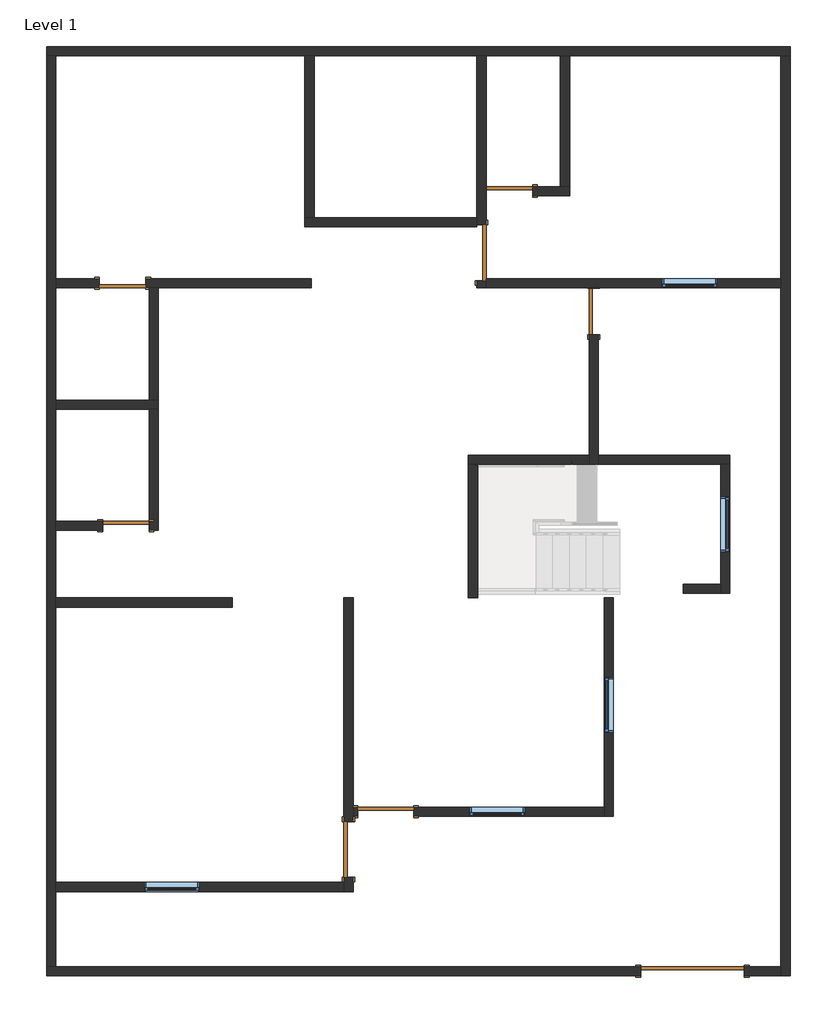
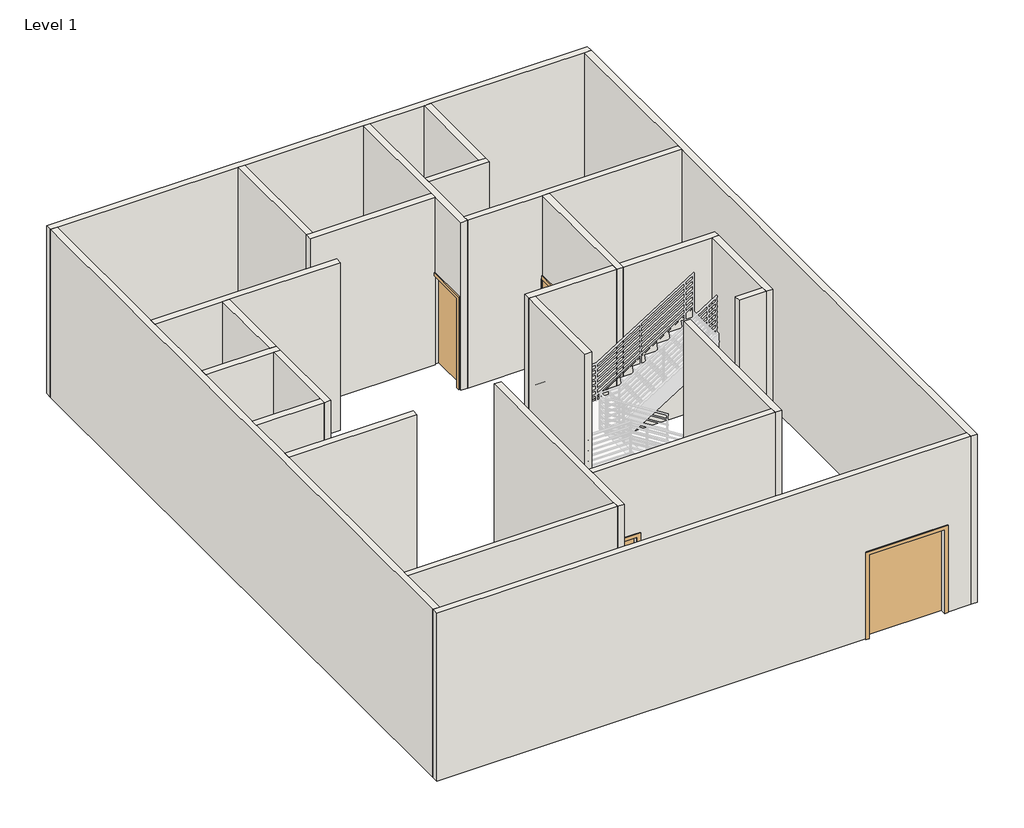
# One storey, part 1 of 4: 26 walls, 8 doors, 5 windows.
"""IFC4 building model written with IfcOpenShell, lengths in millimetres."""

from ifc_helpers import new_model, si_unit, frame, origin, origin_with_axes, place, context, project, spatial, polyline, outline, extrude, faceted_brep, transform, mapped, element, save
from components import m_door_double_flush_panel_double_acting_1700_x_2000mm_42eec5da, m_single_flush_0762_x_2032mm_ffa3ef71, m_single_flush_0762_x_2032mm_3f592dcc, m_single_flush_0915_x_2134mm_138fd904, m_single_flush_0915_x_2134mm_f3d7f739, m_fixed_0915_x_0610mm_ad787ded

model = new_model("IFC4")

# Units and contexts
model_context = context("Model", 3, world=origin())
ifc_project = project(units=[si_unit("LENGTHUNIT", "METRE", prefix="MILLI")], contexts=[model_context])

# Site, building, storey
site = spatial("IfcSite", under=ifc_project)
building = spatial("IfcBuilding", under=site)
storey = spatial("IfcBuildingStorey", under=building, Name="Level 1", Elevation=0.0)

# Doors
placement = place(None, origin())
m_door_double_flush_panel_double_acting_1700_x_2000mm_shape = m_door_double_flush_panel_double_acting_1700_x_2000mm_42eec5da(model_context)
element("IfcDoor", 1, ObjectType="M_Door-Double-Flush_Panel-Double-Acting : 1700 x 2000mm", at=placement, inside=storey, context=model_context, shape_type="MappedRepresentation", body=[
    mapped(m_door_double_flush_panel_double_acting_1700_x_2000mm_shape, transform((658.3084763, -5386.7690536, 0.0), x_axis=(1.0, 0.0, 0.0), y_axis=(0.0, 1.0, 0.0), z_axis=(0.0, 0.0, 1.0))),
])
m_single_flush_0762_x_2032mm_shape = m_single_flush_0762_x_2032mm_ffa3ef71(model_context)
element("IfcDoor", 2, ObjectType="M_Single-Flush : 0762 x 2032mm", at=placement, inside=storey, context=model_context, shape_type="MappedRepresentation", body=[
    mapped(m_single_flush_0762_x_2032mm_shape, transform((-2346.0915237, 7408.1309464, 0.0), x_axis=(-1.0, 0.0, 0.0), y_axis=(0.0, -1.0, 0.0), z_axis=(0.0, 0.0, 1.0))),
])
element("IfcDoor", 3, ObjectType="M_Single-Flush : 0762 x 2032mm", at=placement, inside=storey, context=model_context, shape_type="MappedRepresentation", body=[
    mapped(m_single_flush_0762_x_2032mm_shape, transform((-8686.1415237, 5894.4309464, 0.0), x_axis=(1.0, 0.0, 0.0), y_axis=(0.0, 1.0, 0.0), z_axis=(0.0, 0.0, 1.0))),
])
m_single_flush_0762_x_2032mm_2_shape = m_single_flush_0762_x_2032mm_3f592dcc(model_context)
element("IfcDoor", 4, ObjectType="M_Single-Flush : 0762 x 2032mm", at=placement, inside=storey, context=model_context, shape_type="MappedRepresentation", body=[
    mapped(m_single_flush_0762_x_2032mm_2_shape, transform((-8635.3415237, 1920.5309464, 0.0), x_axis=(1.0, 0.0, 0.0), y_axis=(0.0, 1.0, 0.0), z_axis=(0.0, 0.0, 1.0))),
])
element("IfcDoor", 5, ObjectType="M_Single-Flush : 0762 x 2032mm", at=placement, inside=storey, context=model_context, shape_type="MappedRepresentation", body=[
    mapped(m_single_flush_0762_x_2032mm_2_shape, transform((-962.9915237, 5437.2309464, 0.0), x_axis=(0.0, 1.0, 0.0), y_axis=(-1.0, 0.0, 0.0), z_axis=(0.0, 0.0, 1.0))),
])
m_single_flush_0915_x_2134mm_shape = m_single_flush_0915_x_2134mm_138fd904(model_context)
element("IfcDoor", 6, ObjectType="M_Single-Flush : 0915 x 2134mm", at=placement, inside=storey, context=model_context, shape_type="MappedRepresentation", body=[
    mapped(m_single_flush_0915_x_2134mm_shape, transform((-2803.2915237, 6396.6809464, 0.0), x_axis=(0.0, -1.0, 0.0), y_axis=(1.0, 0.0, 0.0), z_axis=(0.0, 0.0, 1.0))),
])
m_single_flush_0915_x_2134mm_2_shape = m_single_flush_0915_x_2134mm_f3d7f739(model_context)
element("IfcDoor", 7, ObjectType="M_Single-Flush : 0915 x 2134mm", at=placement, inside=storey, context=model_context, shape_type="MappedRepresentation", body=[
    mapped(m_single_flush_0915_x_2134mm_2_shape, transform((-4982.8915237, -3387.7190536, 0.0), x_axis=(0.0, -1.0, 0.0), y_axis=(1.0, 0.0, 0.0), z_axis=(0.0, 0.0, 1.0))),
])
element("IfcDoor", 8, ObjectType="M_Single-Flush : 0915 x 2134mm", at=placement, inside=storey, context=model_context, shape_type="MappedRepresentation", body=[
    mapped(m_single_flush_0915_x_2134mm_2_shape, transform((-4373.2915237, -2771.7690536, 0.0), x_axis=(-1.0, 0.0, 0.0), y_axis=(0.0, -1.0, 0.0), z_axis=(0.0, 0.0, 1.0))),
])

# Walls
element("IfcWall", 9, ObjectType="Generic - 150mm", at=placement, inside=storey, context=model_context, shape_type="Brep", body=[
    faceted_brep([(-9934.6915237, 9628.2309464, 0.0), (-9784.6915237, 9628.2309464, 0.0), (-5698.8915237, 9628.2309464, 0.0), (-5548.8915237, 9628.2309464, 0.0), (-2878.2915237, 9628.2309464, 0.0), (-2728.2915237, 9628.2309464, 0.0), (-1509.0915237, 9628.2309464, 0.0), (-1359.0915237, 9628.2309464, 0.0), (2107.3084763, 9628.2309464, 0.0), (2257.3084763, 9628.2309464, 0.0), (2257.3084763, 9628.2309464, 4000.0), (2107.3084763, 9628.2309464, 4000.0), (-1359.0915237, 9628.2309464, 4000.0), (-1509.0915237, 9628.2309464, 4000.0), (-2728.2915237, 9628.2309464, 4000.0), (-2878.2915237, 9628.2309464, 4000.0), (-5548.8915237, 9628.2309464, 4000.0), (-5698.8915237, 9628.2309464, 4000.0), (-9784.6915237, 9628.2309464, 4000.0), (-9934.6915237, 9628.2309464, 4000.0), (-9934.6915237, 9778.2309464, 0.0), (-9934.6915237, 9778.2309464, 4000.0), (2257.3084763, 9778.2309464, 4000.0), (2257.3084763, 9778.2309464, 0.0)], [[[0, 1, 2, 3, 4, 5, 6, 7, 8, 9, 10, 11, 12, 13, 14, 15, 16, 17, 18, 19]], [[20, 21, 22, 23]], [[9, 8, 7, 6, 5, 4, 3, 2, 1, 0, 20, 23]], [[19, 18, 17, 16, 15, 14, 13, 12, 11, 10, 22, 21]], [[10, 9, 23, 22]], [[0, 19, 21, 20]]]),
])
element("IfcWall", 10, ObjectType="Generic - 150mm", at=placement, inside=storey, context=model_context, shape_type="Brep", body=[
    faceted_brep([(2107.3084763, 9628.2309464, 0.0), (2107.3084763, 5969.4309464, 0.0), (2107.3084763, 5819.4309464, 0.0), (2107.3084763, -5311.7690536, 0.0), (2107.3084763, -5461.7690536, 0.0), (2107.3084763, -5461.7690536, 4000.0), (2107.3084763, -5311.7690536, 4000.0), (2107.3084763, 5819.4309464, 4000.0), (2107.3084763, 5969.4309464, 4000.0), (2107.3084763, 9628.2309464, 4000.0), (2257.3084763, 9628.2309464, 0.0), (2257.3084763, 9628.2309464, 4000.0), (2257.3084763, -5461.7690536, 4000.0), (2257.3084763, -5461.7690536, 0.0)], [[[0, 1, 2, 3, 4, 5, 6, 7, 8, 9]], [[10, 11, 12, 13]], [[4, 3, 2, 1, 0, 10, 13]], [[9, 8, 7, 6, 5, 12, 11]], [[0, 9, 11, 10]], [[5, 4, 13, 12]]]),
])
element("IfcWall", 11, ObjectType="Generic - 150mm", at=placement, inside=storey, context=model_context, shape_type="Brep", body=[
    faceted_brep([(-9934.6915237, -5311.7690536, 4000.0), (-9784.6915237, -5311.7690536, 4000.0), (2107.3084763, -5311.7690536, 4000.0), (2107.3084763, -5311.7690536, 0.0), (1508.3084763, -5311.7690536, 0.0), (1508.3084763, -5311.7690536, 2000.0), (-191.6915237, -5311.7690536, 2000.0), (-191.6915237, -5311.7690536, 0.0), (-9784.6915237, -5311.7690536, 0.0), (-9934.6915237, -5311.7690536, 0.0), (2107.3084763, -5461.7690536, 4000.0), (-9934.6915237, -5461.7690536, 4000.0), (-9934.6915237, -5461.7690536, 0.0), (-191.6915237, -5461.7690536, 0.0), (-191.6915237, -5461.7690536, 2000.0), (1508.3084763, -5461.7690536, 2000.0), (1508.3084763, -5461.7690536, 0.0), (2107.3084763, -5461.7690536, 0.0)], [[[0, 1, 2, 3, 4, 5, 6, 7, 8, 9]], [[10, 11, 12, 13, 14, 15, 16, 17]], [[3, 17, 16, 4]], [[12, 9, 8, 7, 13]], [[2, 1, 0, 11, 10]], [[3, 2, 10, 17]], [[0, 9, 12, 11]], [[15, 5, 4, 16]], [[5, 15, 14, 6]], [[6, 14, 13, 7]]]),
])
element("IfcWall", 12, ObjectType="Generic - 150mm", at=placement, inside=storey, context=model_context, shape_type="Brep", body=[
    faceted_brep([(-9784.6915237, -5311.7690536, 0.0), (-9784.6915237, -4078.6690536, 0.0), (-9784.6915237, -3928.6690536, 0.0), (-9784.6915237, 585.8309464, 0.0), (-9784.6915237, 735.8309464, 0.0), (-9784.6915237, 1845.5309464, 0.0), (-9784.6915237, 1995.5309464, 0.0), (-9784.6915237, 3826.7309464, 0.0), (-9784.6915237, 3976.7309464, 0.0), (-9784.6915237, 5819.4309464, 0.0), (-9784.6915237, 5969.4309464, 0.0), (-9784.6915237, 9628.2309464, 0.0), (-9784.6915237, 9628.2309464, 4000.0), (-9784.6915237, 5969.4309464, 4000.0), (-9784.6915237, 5819.4309464, 4000.0), (-9784.6915237, 3976.7309464, 4000.0), (-9784.6915237, 3826.7309464, 4000.0), (-9784.6915237, 1995.5309464, 4000.0), (-9784.6915237, 1845.5309464, 4000.0), (-9784.6915237, 735.8309464, 4000.0), (-9784.6915237, 585.8309464, 4000.0), (-9784.6915237, -3928.6690536, 4000.0), (-9784.6915237, -4078.6690536, 4000.0), (-9784.6915237, -5311.7690536, 4000.0), (-9934.6915237, -5311.7690536, 0.0), (-9934.6915237, -5311.7690536, 4000.0), (-9934.6915237, 9628.2309464, 4000.0), (-9934.6915237, 9628.2309464, 0.0)], [[[0, 1, 2, 3, 4, 5, 6, 7, 8, 9, 10, 11, 12, 13, 14, 15, 16, 17, 18, 19, 20, 21, 22, 23]], [[24, 25, 26, 27]], [[11, 10, 9, 8, 7, 6, 5, 4, 3, 2, 1, 0, 24, 27]], [[23, 22, 21, 20, 19, 18, 17, 16, 15, 14, 13, 12, 26, 25]], [[12, 11, 27, 26]], [[0, 23, 25, 24]]]),
])
element("IfcWall", 13, ObjectType="Generic - 150mm", at=placement, inside=storey, context=model_context, shape_type="Brep", body=[
    faceted_brep([(-8305.1415237, 5819.4309464, 2032.0), (-8305.1415237, 5819.4309464, 0.0), (-8253.1415237, 5819.4309464, 0.0), (-8103.1415237, 5819.4309464, 0.0), (-5594.8915237, 5819.4309464, 0.0), (-5594.8915237, 5819.4309464, 4000.0), (-8103.1415237, 5819.4309464, 4000.0), (-8253.1415237, 5819.4309464, 4000.0), (-9784.6915237, 5819.4309464, 4000.0), (-9784.6915237, 5819.4309464, 0.0), (-9067.1415237, 5819.4309464, 0.0), (-9067.1415237, 5819.4309464, 2032.0), (-5594.8915237, 5969.4309464, 0.0), (-8305.1415237, 5969.4309464, 0.0), (-8305.1415237, 5969.4309464, 2032.0), (-9067.1415237, 5969.4309464, 2032.0), (-9067.1415237, 5969.4309464, 0.0), (-9784.6915237, 5969.4309464, 0.0), (-9784.6915237, 5969.4309464, 4000.0), (-5594.8915237, 5969.4309464, 4000.0)], [[[0, 1, 2, 3, 4, 5, 6, 7, 8, 9, 10, 11]], [[12, 13, 14, 15, 16, 17, 18, 19]], [[10, 9, 17, 16]], [[4, 3, 2, 1, 13, 12]], [[5, 4, 12, 19]], [[8, 7, 6, 5, 19, 18]], [[9, 8, 18, 17]], [[14, 13, 1, 0]], [[15, 14, 0, 11]], [[16, 15, 11, 10]]]),
])
element("IfcWall", 14, ObjectType="Generic - 150mm", at=placement, inside=storey, context=model_context, shape_type="Brep", body=[
    faceted_brep([(-5698.8915237, 6823.9309464, 0.0), (-2878.2915237, 6823.9309464, 0.0), (-2878.2915237, 6823.9309464, 4000.0), (-5698.8915237, 6823.9309464, 4000.0), (-5698.8915237, 6973.9309464, 0.0), (-5698.8915237, 6973.9309464, 4000.0), (-5548.8915237, 6973.9309464, 4000.0), (-2878.2915237, 6973.9309464, 4000.0), (-2878.2915237, 6973.9309464, 0.0), (-5548.8915237, 6973.9309464, 0.0), (-2878.2915237, 6854.1809464, 0.0)], [[[0, 1, 2, 3]], [[4, 5, 6, 7, 8, 9]], [[1, 0, 4, 9, 8, 10]], [[3, 2, 7, 6, 5]], [[2, 1, 10, 8, 7]], [[0, 3, 5, 4]]]),
])
element("IfcWall", 15, ObjectType="Generic - 150mm", at=placement, inside=storey, context=model_context, shape_type="Brep", body=[
    faceted_brep([(-2728.2915237, 5819.4309464, 0.0), (-2728.2915237, 5939.1809464, 0.0), (-2728.2915237, 5939.1809464, 2134.0), (-2728.2915237, 6854.1809464, 2134.0), (-2728.2915237, 6854.1809464, 0.0), (-2728.2915237, 7333.1309464, 0.0), (-2728.2915237, 7483.1309464, 0.0), (-2728.2915237, 9628.2309464, 0.0), (-2728.2915237, 9628.2309464, 4000.0), (-2728.2915237, 7483.1309464, 4000.0), (-2728.2915237, 7333.1309464, 4000.0), (-2728.2915237, 5969.4309464, 4000.0), (-2728.2915237, 5819.4309464, 4000.0), (-2878.2915237, 5939.1809464, 2134.0), (-2878.2915237, 5939.1809464, 0.0), (-2878.2915237, 5819.4309464, 0.0), (-2878.2915237, 5819.4309464, 4000.0), (-2878.2915237, 6823.9309464, 4000.0), (-2878.2915237, 6973.9309464, 4000.0), (-2878.2915237, 9628.2309464, 4000.0), (-2878.2915237, 9628.2309464, 0.0), (-2878.2915237, 6973.9309464, 0.0), (-2878.2915237, 6854.1809464, 0.0), (-2878.2915237, 6854.1809464, 2134.0)], [[[0, 1, 2, 3, 4, 5, 6, 7, 8, 9, 10, 11, 12]], [[13, 14, 15, 16, 17, 18, 19, 20, 21, 22, 23]], [[15, 14, 1, 0]], [[22, 21, 20, 7, 6, 5, 4]], [[12, 11, 10, 9, 8, 19, 18, 17, 16]], [[8, 7, 20, 19]], [[0, 12, 16, 15]], [[2, 1, 14, 13]], [[3, 2, 13, 23]], [[4, 3, 23, 22]]]),
])
element("IfcWall", 16, ObjectType="Generic - 150mm", at=placement, inside=storey, context=model_context, shape_type="Brep", body=[
    faceted_brep([(-2728.2915237, 7333.1309464, 0.0), (-2727.0915237, 7333.1309464, 0.0), (-2727.0915237, 7333.1309464, 2032.0), (-1965.0915237, 7333.1309464, 2032.0), (-1965.0915237, 7333.1309464, 0.0), (-1359.0915237, 7333.1309464, 0.0), (-1359.0915237, 7333.1309464, 4000.0), (-2728.2915237, 7333.1309464, 4000.0), (-2727.0915237, 7483.1309464, 2032.0), (-2727.0915237, 7483.1309464, 0.0), (-2728.2915237, 7483.1309464, 0.0), (-2728.2915237, 7483.1309464, 4000.0), (-1509.0915237, 7483.1309464, 4000.0), (-1359.0915237, 7483.1309464, 4000.0), (-1359.0915237, 7483.1309464, 0.0), (-1509.0915237, 7483.1309464, 0.0), (-1965.0915237, 7483.1309464, 0.0), (-1965.0915237, 7483.1309464, 2032.0)], [[[0, 1, 2, 3, 4, 5, 6, 7]], [[8, 9, 10, 11, 12, 13, 14, 15, 16, 17]], [[10, 9, 1, 0]], [[16, 15, 14, 5, 4]], [[7, 6, 13, 12, 11]], [[0, 7, 11, 10]], [[6, 5, 14, 13]], [[2, 1, 9, 8]], [[3, 2, 8, 17]], [[4, 3, 17, 16]]]),
])
element("IfcWall", 17, ObjectType="Generic - 150mm", at=placement, inside=storey, context=model_context, shape_type="SweptSolid", body=[
    extrude(outline(polyline([(-1359.0915237, 9628.2309464), (-1359.0915237, 7483.1309464), (-1509.0915237, 7483.1309464), (-1509.0915237, 9628.2309464), (-1359.0915237, 9628.2309464)])), origin_with_axes(), (0.0, 0.0, 1.0), 4000.0),
])
element("IfcWall", 18, ObjectType="Generic - 150mm", at=placement, inside=storey, context=model_context, shape_type="Brep", body=[
    faceted_brep([(2107.3084763, 5969.4309464, 0.0), (-2728.2915237, 5969.4309464, 0.0), (-2728.2915237, 5969.4309464, 4000.0), (2107.3084763, 5969.4309464, 4000.0), (1067.1584763, 5969.4309464, 915.0), (1067.1584763, 5969.4309464, 1525.0), (152.1584763, 5969.4309464, 1525.0), (152.1584763, 5969.4309464, 915.0), (2107.3084763, 5819.4309464, 0.0), (2107.3084763, 5819.4309464, 4000.0), (-887.9915237, 5819.4309464, 4000.0), (-1037.9915237, 5819.4309464, 4000.0), (-2728.2915237, 5819.4309464, 4000.0), (-2728.2915237, 5819.4309464, 0.0), (-1037.9915237, 5819.4309464, 0.0), (-887.9915237, 5819.4309464, 0.0), (1067.1584763, 5819.4309464, 915.0), (152.1584763, 5819.4309464, 915.0), (152.1584763, 5819.4309464, 1525.0), (1067.1584763, 5819.4309464, 1525.0), (-2728.2915237, 5939.1809464, 0.0)], [[[0, 1, 2, 3], [4, 5, 6, 7]], [[8, 9, 10, 11, 12, 13, 14, 15], [16, 17, 18, 19]], [[1, 0, 8, 15, 14, 13, 20]], [[3, 2, 12, 11, 10, 9]], [[0, 3, 9, 8]], [[2, 1, 20, 13, 12]], [[5, 4, 16, 19]], [[6, 5, 19, 18]], [[7, 6, 18, 17]], [[4, 7, 17, 16]]]),
])
element("IfcWall", 19, ObjectType="Generic - 150mm", at=placement, inside=storey, context=model_context, shape_type="SweptSolid", body=[
    extrude(outline(polyline([(-5698.8915237, 6973.9309464), (-5698.8915237, 9628.2309464), (-5548.8915237, 9628.2309464), (-5548.8915237, 6973.9309464), (-5698.8915237, 6973.9309464)])), origin_with_axes(), (0.0, 0.0, 1.0), 4000.0),
])
element("IfcWall", 20, ObjectType="Generic - 150mm", at=placement, inside=storey, context=model_context, shape_type="Brep", body=[
    faceted_brep([(-9784.6915237, 3826.7309464, 0.0), (-8253.1415237, 3826.7309464, 0.0), (-8103.1415237, 3826.7309464, 0.0), (-8103.1415237, 3826.7309464, 4000.0), (-8253.1415237, 3826.7309464, 4000.0), (-9784.6915237, 3826.7309464, 4000.0), (-9784.6915237, 3976.7309464, 0.0), (-9784.6915237, 3976.7309464, 4000.0), (-8253.1415237, 3976.7309464, 4000.0), (-8103.1415237, 3976.7309464, 4000.0), (-8103.1415237, 3976.7309464, 0.0), (-8253.1415237, 3976.7309464, 0.0)], [[[0, 1, 2, 3, 4, 5]], [[6, 7, 8, 9, 10, 11]], [[2, 1, 0, 6, 11, 10]], [[5, 4, 3, 9, 8, 7]], [[0, 5, 7, 6]], [[3, 2, 10, 9]]]),
])
element("IfcWall", 21, ObjectType="Generic - 150mm", at=placement, inside=storey, context=model_context, shape_type="SweptSolid", body=[
    extrude(outline(polyline([(-8103.1415237, 5819.4309464), (-8103.1415237, 3976.7309464), (-8253.1415237, 3976.7309464), (-8253.1415237, 5819.4309464), (-8103.1415237, 5819.4309464)])), origin_with_axes(), (0.0, 0.0, 1.0), 4000.0),
])
element("IfcWall", 22, ObjectType="Generic - 150mm", at=placement, inside=storey, context=model_context, shape_type="Brep", body=[
    faceted_brep([(-8253.1415237, 3826.7309464, 0.0), (-8253.1415237, 1995.5309464, 0.0), (-8253.1415237, 1845.5309464, 0.0), (-8253.1415237, 1845.5309464, 4000.0), (-8253.1415237, 1995.5309464, 4000.0), (-8253.1415237, 3826.7309464, 4000.0), (-8103.1415237, 3826.7309464, 0.0), (-8103.1415237, 3826.7309464, 4000.0), (-8103.1415237, 1845.5309464, 4000.0), (-8103.1415237, 1845.5309464, 0.0)], [[[0, 1, 2, 3, 4, 5]], [[6, 7, 8, 9]], [[2, 1, 0, 6, 9]], [[5, 4, 3, 8, 7]], [[0, 5, 7, 6]], [[3, 2, 9, 8]]]),
])
element("IfcWall", 23, ObjectType="Generic - 150mm", at=placement, inside=storey, context=model_context, shape_type="SweptSolid", body=[
    extrude(outline(polyline([(2032.0, -8254.3415237), (0.0, -8254.3415237), (0.0, -8253.1415237), (4000.0, -8253.1415237), (4000.0, -9784.6915237), (0.0, -9784.6915237), (0.0, -9016.3415237), (2032.0, -9016.3415237), (2032.0, -8254.3415237)])), frame((0.0, 1845.5309464, 0.0), z_axis=(0.0, 1.0, 0.0), x_axis=(0.0, 0.0, 1.0)), (0.0, 0.0, 1.0), 150.0),
])
element("IfcWall", 24, ObjectType="Generic - 150mm", at=placement, inside=storey, context=model_context, shape_type="Brep", body=[
    faceted_brep([(-1037.9915237, 5819.4309464, 0.0), (-1037.9915237, 5818.2309464, 0.0), (-1037.9915237, 5818.2309464, 2032.0), (-1037.9915237, 5056.2309464, 2032.0), (-1037.9915237, 5056.2309464, 0.0), (-1037.9915237, 3076.2309464, 0.0), (-1037.9915237, 2926.2309464, 0.0), (-1037.9915237, 2926.2309464, 4000.0), (-1037.9915237, 3076.2309464, 4000.0), (-1037.9915237, 5819.4309464, 4000.0), (-887.9915237, 5818.2309464, 2032.0), (-887.9915237, 5818.2309464, 0.0), (-887.9915237, 5819.4309464, 0.0), (-887.9915237, 5819.4309464, 4000.0), (-887.9915237, 3076.2309464, 4000.0), (-887.9915237, 2926.2309464, 4000.0), (-887.9915237, 2926.2309464, 0.0), (-887.9915237, 3076.2309464, 0.0), (-887.9915237, 5056.2309464, 0.0), (-887.9915237, 5056.2309464, 2032.0)], [[[0, 1, 2, 3, 4, 5, 6, 7, 8, 9]], [[10, 11, 12, 13, 14, 15, 16, 17, 18, 19]], [[12, 11, 1, 0]], [[18, 17, 16, 6, 5, 4]], [[9, 8, 7, 15, 14, 13]], [[0, 9, 13, 12]], [[7, 6, 16, 15]], [[2, 1, 11, 10]], [[3, 2, 10, 19]], [[4, 3, 19, 18]]]),
])
element("IfcWall", 25, ObjectType="Generic - 150mm", at=placement, inside=storey, context=model_context, shape_type="Brep", body=[
    faceted_brep([(-887.9915237, 2926.2309464, 0.0), (1117.9084763, 2926.2309464, 0.0), (1267.9084763, 2926.2309464, 0.0), (1267.9084763, 2926.2309464, 4000.0), (1117.9084763, 2926.2309464, 4000.0), (-887.9915237, 2926.2309464, 4000.0), (-887.9915237, 3076.2309464, 0.0), (-887.9915237, 3076.2309464, 4000.0), (1267.9084763, 3076.2309464, 4000.0), (1267.9084763, 3076.2309464, 0.0)], [[[0, 1, 2, 3, 4, 5]], [[6, 7, 8, 9]], [[2, 1, 0, 6, 9]], [[5, 4, 3, 8, 7]], [[0, 5, 7, 6]], [[3, 2, 9, 8]]]),
])
element("IfcWall", 26, ObjectType="Generic - 150mm", at=placement, inside=storey, context=model_context, shape_type="Brep", body=[
    faceted_brep([(-5057.8915237, -3845.2190536, 2134.0), (-5057.8915237, -3845.2190536, 0.0), (-5057.8915237, -3928.6690536, 0.0), (-5057.8915237, -4078.6690536, 0.0), (-5057.8915237, -4078.6690536, 4000.0), (-5057.8915237, -3928.6690536, 4000.0), (-5057.8915237, 735.8309464, 4000.0), (-5057.8915237, 735.8309464, 0.0), (-5057.8915237, -2930.2190536, 0.0), (-5057.8915237, -2930.2190536, 2134.0), (-4907.8915237, -4078.6690536, 0.0), (-4907.8915237, -3845.2190536, 0.0), (-4907.8915237, -3845.2190536, 2134.0), (-4907.8915237, -2930.2190536, 2134.0), (-4907.8915237, -2930.2190536, 0.0), (-4907.8915237, -2846.7690536, 0.0), (-4907.8915237, -2696.7690536, 0.0), (-4907.8915237, 735.8309464, 0.0), (-4907.8915237, 735.8309464, 4000.0), (-4907.8915237, -2696.7690536, 4000.0), (-4907.8915237, -2846.7690536, 4000.0), (-4907.8915237, -4078.6690536, 4000.0)], [[[0, 1, 2, 3, 4, 5, 6, 7, 8, 9]], [[10, 11, 12, 13, 14, 15, 16, 17, 18, 19, 20, 21]], [[8, 7, 17, 16, 15, 14]], [[3, 2, 1, 11, 10]], [[6, 5, 4, 21, 20, 19, 18]], [[7, 6, 18, 17]], [[4, 3, 10, 21]], [[12, 11, 1, 0]], [[13, 12, 0, 9]], [[14, 13, 9, 8]]]),
])
element("IfcWall", 27, ObjectType="Generic - 150mm", at=placement, inside=storey, context=model_context, shape_type="SweptSolid", body=[
    extrude(outline(polyline([(0.0, -5057.8915237), (4000.0, -5057.8915237), (4000.0, -9784.6915237), (0.0, -9784.6915237), (0.0, -5057.8915237)]), holes=[polyline([(915.0, -7420.9915237), (915.0, -8335.9915237), (1525.0, -8335.9915237), (1525.0, -7420.9915237), (915.0, -7420.9915237)])]), frame((0.0, -4078.6690536, 0.0), z_axis=(0.0, 1.0, 0.0), x_axis=(0.0, 0.0, 1.0)), (0.0, 0.0, 1.0), 150.0),
])
element("IfcWall", 28, ObjectType="Generic - 150mm", at=placement, inside=storey, context=model_context, shape_type="Brep", body=[
    faceted_brep([(-790.6915237, 735.8309464, 0.0), (-790.6915237, -2696.7690536, 0.0), (-790.6915237, -2846.7690536, 0.0), (-790.6915237, -2846.7690536, 4000.0), (-790.6915237, -2696.7690536, 4000.0), (-790.6915237, 735.8309464, 4000.0), (-790.6915237, -1475.4690536, 915.0), (-790.6915237, -560.4690536, 915.0), (-790.6915237, -560.4690536, 1525.0), (-790.6915237, -1475.4690536, 1525.0), (-640.6915237, 735.8309464, 0.0), (-640.6915237, 735.8309464, 4000.0), (-640.6915237, -2846.7690536, 4000.0), (-640.6915237, -2846.7690536, 0.0), (-640.6915237, -1475.4690536, 915.0), (-640.6915237, -1475.4690536, 1525.0), (-640.6915237, -560.4690536, 1525.0), (-640.6915237, -560.4690536, 915.0)], [[[0, 1, 2, 3, 4, 5], [6, 7, 8, 9]], [[10, 11, 12, 13], [14, 15, 16, 17]], [[2, 1, 0, 10, 13]], [[5, 4, 3, 12, 11]], [[0, 5, 11, 10]], [[3, 2, 13, 12]], [[15, 14, 6, 9]], [[16, 15, 9, 8]], [[17, 16, 8, 7]], [[14, 17, 7, 6]]]),
])
element("IfcWall", 29, ObjectType="Generic - 150mm", at=placement, inside=storey, context=model_context, shape_type="SweptSolid", body=[
    extrude(outline(polyline([(0.0, -4907.8915237), (0.0, -4830.7915237), (2134.0, -4830.7915237), (2134.0, -3915.7915237), (0.0, -3915.7915237), (0.0, -790.6915237), (4000.0, -790.6915237), (4000.0, -4907.8915237), (0.0, -4907.8915237)]), holes=[polyline([(915.0, -2086.9915237), (915.0, -3001.9915237), (1525.0, -3001.9915237), (1525.0, -2086.9915237), (915.0, -2086.9915237)])]), frame((0.0, -2846.7690536, 0.0), z_axis=(0.0, 1.0, 0.0), x_axis=(0.0, 0.0, 1.0)), (0.0, 0.0, 1.0), 150.0),
])
element("IfcWall", 30, ObjectType="Generic - 150mm", at=placement, inside=storey, context=model_context, shape_type="Brep", body=[
    faceted_brep([(-1037.9915237, 3076.2309464, 0.0), (-3016.7915237, 3076.2309464, 0.0), (-3016.7915237, 3076.2309464, 4000.0), (-1037.9915237, 3076.2309464, 4000.0), (-1037.9915237, 2926.2309464, 0.0), (-1037.9915237, 2926.2309464, 4000.0), (-2866.7915237, 2926.2309464, 4000.0), (-3016.7915237, 2926.2309464, 4000.0), (-3016.7915237, 2926.2309464, 0.0), (-2866.7915237, 2926.2309464, 0.0)], [[[0, 1, 2, 3]], [[4, 5, 6, 7, 8, 9]], [[1, 0, 4, 9, 8]], [[3, 2, 7, 6, 5]], [[0, 3, 5, 4]], [[2, 1, 8, 7]]]),
])
element("IfcWall", 31, ObjectType="Generic - 150mm", at=placement, inside=storey, context=model_context, shape_type="SweptSolid", body=[
    extrude(outline(polyline([(-3016.7915237, 735.8309464), (-3016.7915237, 2926.2309464), (-2866.7915237, 2926.2309464), (-2866.7915237, 735.8309464), (-3016.7915237, 735.8309464)])), origin_with_axes(), (0.0, 0.0, 1.0), 4000.0),
])
element("IfcWall", 32, ObjectType="Generic - 150mm", at=placement, inside=storey, context=model_context, shape_type="Brep", body=[
    faceted_brep([(1117.9084763, 2926.2309464, 0.0), (1117.9084763, 960.8309464, 0.0), (1117.9084763, 810.8309464, 0.0), (1117.9084763, 810.8309464, 4000.0), (1117.9084763, 960.8309464, 4000.0), (1117.9084763, 2926.2309464, 4000.0), (1117.9084763, 2401.0309464, 915.0), (1117.9084763, 2401.0309464, 1525.0), (1117.9084763, 1486.0309464, 1525.0), (1117.9084763, 1486.0309464, 915.0), (1267.9084763, 2926.2309464, 0.0), (1267.9084763, 2926.2309464, 4000.0), (1267.9084763, 810.8309464, 4000.0), (1267.9084763, 810.8309464, 0.0), (1267.9084763, 2401.0309464, 915.0), (1267.9084763, 1486.0309464, 915.0), (1267.9084763, 1486.0309464, 1525.0), (1267.9084763, 2401.0309464, 1525.0)], [[[0, 1, 2, 3, 4, 5], [6, 7, 8, 9]], [[10, 11, 12, 13], [14, 15, 16, 17]], [[2, 1, 0, 10, 13]], [[5, 4, 3, 12, 11]], [[3, 2, 13, 12]], [[0, 5, 11, 10]], [[7, 6, 14, 17]], [[8, 7, 17, 16]], [[9, 8, 16, 15]], [[6, 9, 15, 14]]]),
])
element("IfcWall", 33, ObjectType="Generic - 150mm", at=placement, inside=storey, context=model_context, shape_type="SweptSolid", body=[
    extrude(outline(polyline([(505.9084763, 960.8309464), (1117.9084763, 960.8309464), (1117.9084763, 810.8309464), (505.9084763, 810.8309464), (505.9084763, 960.8309464)])), origin_with_axes(), (0.0, 0.0, 1.0), 4000.0),
])
element("IfcWall", 34, ObjectType="Generic - 150mm", at=placement, inside=storey, context=model_context, shape_type="SweptSolid", body=[
    extrude(outline(polyline([(-6889.0915237, 585.8309464), (-9784.6915237, 585.8309464), (-9784.6915237, 735.8309464), (-6889.0915237, 735.8309464), (-6889.0915237, 585.8309464)])), origin_with_axes(), (0.0, 0.0, 1.0), 4000.0),
])

# Windows
m_fixed_0915_x_0610mm_shape = m_fixed_0915_x_0610mm_ad787ded(model_context)
element("IfcWindow", 35, ObjectType="M_Fixed : 0915 x 0610mm", at=placement, inside=storey, context=model_context, shape_type="MappedRepresentation", body=[
    mapped(m_fixed_0915_x_0610mm_shape, transform((-7878.4915237, -3990.6690536, 0.0), x_axis=(-1.0, 0.0, 0.0), y_axis=(0.0, -1.0, 0.0), z_axis=(0.0, 0.0, 1.0))),
])
element("IfcWindow", 36, ObjectType="M_Fixed : 0915 x 0610mm", at=placement, inside=storey, context=model_context, shape_type="MappedRepresentation", body=[
    mapped(m_fixed_0915_x_0610mm_shape, transform((-2544.4915237, -2758.7690536, 0.0), x_axis=(-1.0, 0.0, 0.0), y_axis=(0.0, -1.0, 0.0), z_axis=(0.0, 0.0, 1.0))),
])
element("IfcWindow", 37, ObjectType="M_Fixed : 0915 x 0610mm", at=placement, inside=storey, context=model_context, shape_type="MappedRepresentation", body=[
    mapped(m_fixed_0915_x_0610mm_shape, transform((-702.6915237, -1017.9690536, 0.0), x_axis=(0.0, 1.0, 0.0), y_axis=(-1.0, 0.0, 0.0), z_axis=(0.0, 0.0, 1.0))),
])
element("IfcWindow", 38, ObjectType="M_Fixed : 0915 x 0610mm", at=placement, inside=storey, context=model_context, shape_type="MappedRepresentation", body=[
    mapped(m_fixed_0915_x_0610mm_shape, transform((1179.9084763, 1943.5309464, 0.0), x_axis=(0.0, -1.0, 0.0), y_axis=(1.0, 0.0, 0.0), z_axis=(0.0, 0.0, 1.0))),
])
element("IfcWindow", 39, ObjectType="M_Fixed : 0915 x 0610mm", at=placement, inside=storey, context=model_context, shape_type="MappedRepresentation", body=[
    mapped(m_fixed_0915_x_0610mm_shape, transform((609.6584763, 5907.4309464, 0.0), x_axis=(-1.0, 0.0, 0.0), y_axis=(0.0, -1.0, 0.0), z_axis=(0.0, 0.0, 1.0))),
])

save(model, "model.ifc")

# Revit data of these elements
# Type "M_Door-Double-Flush_Panel-Double-Acting : 1700 x 2000mm"
#   Type Mark = "22"
#   Construction Type Id = "DOOR"
#   Assembly Code = "C1020"
#   Analytic Construction = "Wooden"
#   W = 850 mm
#   Thickness = 50 mm
#   Thermal Resistance (R) = 0.455703 (m²·K)/W
#   Swing Angle [instance default] = 90.00°
#   Heat Transfer Coefficient (U) = 2.19465 W/(m²·K)
#   Height = 2000 mm
#   Trim Projection Ext. = 25 mm
#   Trim Projection Int. = 25 mm
#   Trim Width Ext. = 80 mm
#   Trim Width Int. = 80 mm
#   Width = 1700 mm
#   Define Thermal Properties by = 1
#   Panel Material = Wood - Birch - Solid Stained Light Low Gloss
#   Trim Material = Paint - Sienna
#   Visual Light Transmittance = 0
#   Solar Heat Gain Coefficient = 0
#   Function = (empty or 0)
#   Wall Closure = (empty or 0)
# Type "M_Single-Flush : 0762 x 2032mm"
#   Type Mark = "19"
#   Thickness = 51 mm
#   Height = 2032 mm
#   Trim Projection Ext = 25 mm
#   Trim Projection Int = 25 mm
#   Trim Width = 76 mm
#   Width = 762 mm
#   Door Material = Door - Panel
#   Frame Material = Door - Frame
#   Function = (empty or 0)
#   Wall Closure = (empty or 0)
# Type "M_Single-Flush : 0915 x 2134mm"
#   Type Mark = "15"
#   Thickness = 51 mm
#   Height = 2134 mm
#   Trim Projection Ext = 25 mm
#   Trim Projection Int = 25 mm
#   Trim Width = 76 mm
#   Width = 915 mm
#   Door Material = Door - Panel
#   Frame Material = Door - Frame
#   Function = (empty or 0)
#   Wall Closure = (empty or 0)
# Type "Generic - 150mm"
#   Layers, outside or top first: 150 mm no material (function 1)
# Type "M_Fixed : 0915 x 0610mm"
#   Type Mark = "14"
#   Height = 610 mm
#   Default Sill Height = 915 mm
#   Width = 915 mm
#   Window Inset = 19 mm
#   Frame Exterior Material = Sash
#   Frame Interior Material = Sash
#   Glass Pane Material = Glass
#   Sash = Sash
#   Wall Closure = (empty or 0)
# Element 1 (IfcDoor, "M_Door-Double-Flush_Panel-Double-Acting : 1700 x 2000mm")
#   Swing Angle = 90.00°
#   Phase Created = New Construction
#   Materials on its faces: "Paint - Sienna", "Wood - Birch - Solid Stained Light Low Gloss"
# Elements 2, 3, 4, 5 (IfcDoor, "M_Single-Flush : 0762 x 2032mm")
#   Phase Created = New Construction
#   Materials on its faces: "Door - Frame", "Door - Panel"
# Elements 6, 7, 8 (IfcDoor, "M_Single-Flush : 0915 x 2134mm")
#   Phase Created = New Construction
#   Materials on its faces: "Door - Frame", "Door - Panel"
# Elements 9, 10, 11, 12, 13, 14, 15, 16, 17, 18, 19, 20, 21, 22, 23, 24, 25, 26, 27, 28, 29, 30, 31, 32, 33, 34 (IfcWall, "Generic - 150mm")
#   Top Offset = 0 mm
#   Base Offset = 0 mm
#   wall height = 4000 mm
#   Phase Created = New Construction
#   Base Constraint = Level 1
#   Top Constraint = Level 2
#   Materials on its faces: "Default Wall"
# Element 35 (IfcWindow, "M_Fixed : 0915 x 0610mm")
#   Mark = "6"
#   Phase Created = New Construction
#   Materials on its faces: "Sash", "Glass"
# Element 36 (IfcWindow, "M_Fixed : 0915 x 0610mm")
#   Mark = "7"
#   Phase Created = New Construction
#   Materials on its faces: "Sash", "Glass"
# Element 37 (IfcWindow, "M_Fixed : 0915 x 0610mm")
#   Mark = "8"
#   Phase Created = New Construction
#   Materials on its faces: "Sash", "Glass"
# Element 38 (IfcWindow, "M_Fixed : 0915 x 0610mm")
#   Mark = "9"
#   Phase Created = New Construction
#   Materials on its faces: "Sash", "Glass"
# Element 39 (IfcWindow, "M_Fixed : 0915 x 0610mm")
#   Mark = "10"
#   Phase Created = New Construction
#   Materials on its faces: "Sash", "Glass"
# Materials
#   "Wood - Birch - Solid Stained Light Low Gloss": class "Wood", colour RGB 210 159 95, transparency 0, Cost = 0
#   "Paint - Sienna": colour RGB 118 70 51, transparency 0, Cost = 0
#   "Door - Panel": class "Wood", colour RGB 114 82 51, transparency 0
#   "Door - Frame": colour RGB 153 76 43, transparency 0
#   "Sash": class "Wood", colour RGB 136 99 55, transparency 0
#   "Glass": class "Glass", colour RGB 218 227 224, transparency 0.85, Description = "Soda Lime Glass", Cost = 0
#   "Default Wall": colour RGB 80 80 80, transparency 0
